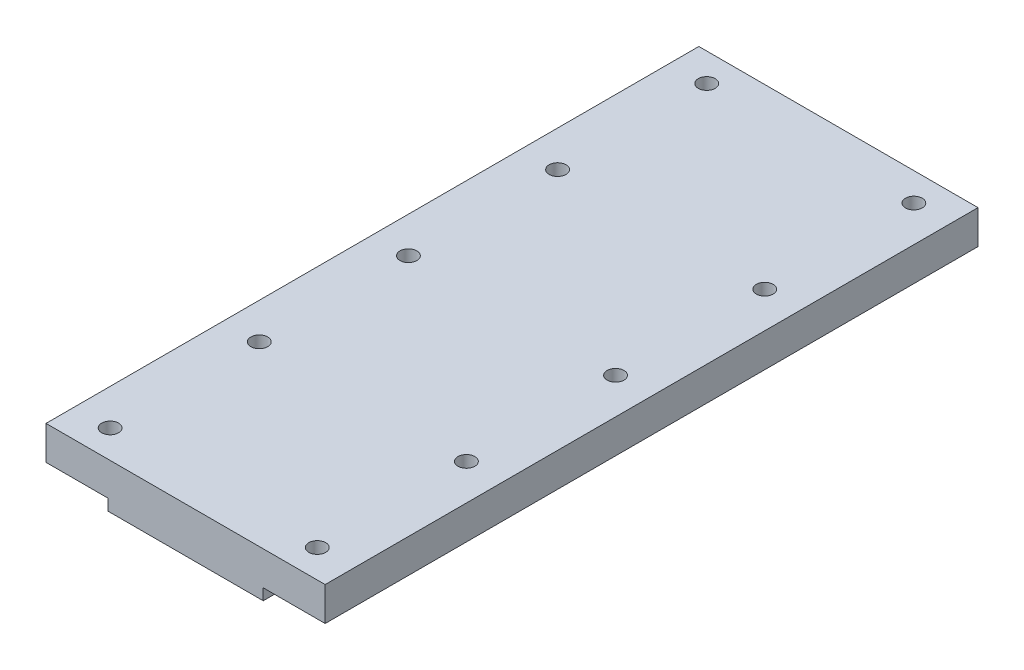
ISO-10303-21;
HEADER;
FILE_DESCRIPTION(('STEP AP214'),'2;1');
FILE_NAME('part.step','',(''),(''),'','','');
FILE_SCHEMA(('AUTOMOTIVE_DESIGN { 1 0 10303 214 1 1 1 1 }'));
ENDSEC;
DATA;
#1=APPLICATION_CONTEXT('core data for automotive mechanical design processes');
#2=APPLICATION_PROTOCOL_DEFINITION('international standard','automotive_design',2000,#1);
#3=PRODUCT_CONTEXT('',#1,'mechanical');
#4=PRODUCT('Part','Part','',(#3));
#5=PRODUCT_RELATED_PRODUCT_CATEGORY('part','',(#4));
#6=PRODUCT_DEFINITION_FORMATION('','',#4);
#7=PRODUCT_DEFINITION_CONTEXT('part definition',#1,'design');
#8=PRODUCT_DEFINITION('design','',#6,#7);
#9=PRODUCT_DEFINITION_SHAPE('','',#8);
#10=(LENGTH_UNIT() NAMED_UNIT(*) SI_UNIT(.MILLI.,.METRE.));
#11=(NAMED_UNIT(*) PLANE_ANGLE_UNIT() SI_UNIT($,.RADIAN.));
#12=(NAMED_UNIT(*) SI_UNIT($,.STERADIAN.) SOLID_ANGLE_UNIT());
#13=UNCERTAINTY_MEASURE_WITH_UNIT(LENGTH_MEASURE(1.E-05),#10,'distance_accuracy_value','');
#14=(GEOMETRIC_REPRESENTATION_CONTEXT(3) GLOBAL_UNCERTAINTY_ASSIGNED_CONTEXT((#13)) GLOBAL_UNIT_ASSIGNED_CONTEXT((#10,
#11,#12)) REPRESENTATION_CONTEXT('',''));
#15=CARTESIAN_POINT('',(0.,0.,0.));
#16=DIRECTION('',(0.,0.,1.));
#17=DIRECTION('',(1.,0.,0.));
#18=AXIS2_PLACEMENT_3D('',#15,#16,#17);
#19=CARTESIAN_POINT('',(-124.,30.,290.));
#20=DIRECTION('',(1.,0.,0.));
#21=DIRECTION('',(0.,0.,-1.));
#22=AXIS2_PLACEMENT_3D('',#19,#20,#21);
#23=PLANE('',#22);
#24=DIRECTION('',(0.,-1.,0.));
#25=VECTOR('',#24,1.);
#26=CARTESIAN_POINT('',(-124.,30.,-290.));
#27=LINE('',#26,#25);
#28=CARTESIAN_POINT('',(-124.,30.,-290.));
#29=VERTEX_POINT('',#28);
#30=CARTESIAN_POINT('',(-124.,0.,-290.));
#31=VERTEX_POINT('',#30);
#32=EDGE_CURVE('E136',#29,#31,#27,.T.);
#33=ORIENTED_EDGE('',*,*,#32,.T.);
#34=DIRECTION('',(0.,0.,-1.));
#35=VECTOR('',#34,1.);
#36=CARTESIAN_POINT('',(-124.,0.,290.));
#37=LINE('',#36,#35);
#38=CARTESIAN_POINT('',(-124.,0.,290.));
#39=VERTEX_POINT('',#38);
#40=EDGE_CURVE('E11',#39,#31,#37,.T.);
#41=ORIENTED_EDGE('',*,*,#40,.F.);
#42=DIRECTION('',(0.,-1.,0.));
#43=VECTOR('',#42,1.);
#44=CARTESIAN_POINT('',(-124.,30.,290.));
#45=LINE('',#44,#43);
#46=CARTESIAN_POINT('',(-124.,30.,290.));
#47=VERTEX_POINT('',#46);
#48=EDGE_CURVE('E155',#47,#39,#45,.T.);
#49=ORIENTED_EDGE('',*,*,#48,.F.);
#50=DIRECTION('',(0.,0.,-1.));
#51=VECTOR('',#50,1.);
#52=CARTESIAN_POINT('',(-124.,30.,290.));
#53=LINE('',#52,#51);
#54=EDGE_CURVE('E134',#47,#29,#53,.T.);
#55=ORIENTED_EDGE('',*,*,#54,.T.);
#56=EDGE_LOOP('',(#33,#41,#49,#55));
#57=FACE_BOUND('',#56,.T.);
#58=ADVANCED_FACE('F39',(#57),#23,.F.);
#59=CARTESIAN_POINT('',(-124.,0.,290.));
#60=DIRECTION('',(0.,1.,0.));
#61=DIRECTION('',(-1.,0.,0.));
#62=AXIS2_PLACEMENT_3D('',#59,#60,#61);
#63=PLANE('',#62);
#64=CARTESIAN_POINT('',(-92.,0.,265.));
#65=DIRECTION('',(0.,1.,0.));
#66=DIRECTION('',(-1.,0.,0.));
#67=AXIS2_PLACEMENT_3D('',#64,#65,#66);
#68=CIRCLE('',#67,7.50000000000001);
#69=CARTESIAN_POINT('',(-99.5,0.,265.));
#70=VERTEX_POINT('',#69);
#71=EDGE_CURVE('E182',#70,#70,#68,.T.);
#72=ORIENTED_EDGE('',*,*,#71,.T.);
#73=EDGE_LOOP('',(#72));
#74=FACE_BOUND('',#73,.T.);
#75=CARTESIAN_POINT('',(-92.,0.,132.5));
#76=DIRECTION('',(0.,1.,0.));
#77=DIRECTION('',(-1.,0.,0.));
#78=AXIS2_PLACEMENT_3D('',#75,#76,#77);
#79=CIRCLE('',#78,7.50000000000001);
#80=CARTESIAN_POINT('',(-99.5,0.,132.5));
#81=VERTEX_POINT('',#80);
#82=EDGE_CURVE('E177',#81,#81,#79,.T.);
#83=ORIENTED_EDGE('',*,*,#82,.T.);
#84=EDGE_LOOP('',(#83));
#85=FACE_BOUND('',#84,.T.);
#86=CARTESIAN_POINT('',(-92.,0.,0.));
#87=DIRECTION('',(0.,1.,0.));
#88=DIRECTION('',(-1.,0.,0.));
#89=AXIS2_PLACEMENT_3D('',#86,#87,#88);
#90=CIRCLE('',#89,7.50000000000001);
#91=CARTESIAN_POINT('',(-99.5,0.,0.));
#92=VERTEX_POINT('',#91);
#93=EDGE_CURVE('E174',#92,#92,#90,.T.);
#94=ORIENTED_EDGE('',*,*,#93,.T.);
#95=EDGE_LOOP('',(#94));
#96=FACE_BOUND('',#95,.T.);
#97=CARTESIAN_POINT('',(-92.,0.,-132.5));
#98=DIRECTION('',(0.,1.,0.));
#99=DIRECTION('',(-1.,0.,0.));
#100=AXIS2_PLACEMENT_3D('',#97,#98,#99);
#101=CIRCLE('',#100,7.50000000000001);
#102=CARTESIAN_POINT('',(-99.5,0.,-132.5));
#103=VERTEX_POINT('',#102);
#104=EDGE_CURVE('E171',#103,#103,#101,.T.);
#105=ORIENTED_EDGE('',*,*,#104,.T.);
#106=EDGE_LOOP('',(#105));
#107=FACE_BOUND('',#106,.T.);
#108=CARTESIAN_POINT('',(-92.,0.,-265.));
#109=DIRECTION('',(0.,1.,0.));
#110=DIRECTION('',(-1.,0.,0.));
#111=AXIS2_PLACEMENT_3D('',#108,#109,#110);
#112=CIRCLE('',#111,7.50000000000001);
#113=CARTESIAN_POINT('',(-99.5,0.,-265.));
#114=VERTEX_POINT('',#113);
#115=EDGE_CURVE('E170',#114,#114,#112,.T.);
#116=ORIENTED_EDGE('',*,*,#115,.T.);
#117=EDGE_LOOP('',(#116));
#118=FACE_BOUND('',#117,.T.);
#119=DIRECTION('',(1.,0.,0.));
#120=VECTOR('',#119,1.);
#121=CARTESIAN_POINT('',(-124.,0.,-290.));
#122=LINE('',#121,#120);
#123=CARTESIAN_POINT('',(-69.,0.,-290.));
#124=VERTEX_POINT('',#123);
#125=EDGE_CURVE('E137',#31,#124,#122,.T.);
#126=ORIENTED_EDGE('',*,*,#125,.T.);
#127=DIRECTION('',(0.,0.,-1.));
#128=VECTOR('',#127,1.);
#129=CARTESIAN_POINT('',(-69.,0.,290.));
#130=LINE('',#129,#128);
#131=CARTESIAN_POINT('',(-69.,0.,290.));
#132=VERTEX_POINT('',#131);
#133=EDGE_CURVE('E48',#132,#124,#130,.T.);
#134=ORIENTED_EDGE('',*,*,#133,.F.);
#135=DIRECTION('',(1.,0.,0.));
#136=VECTOR('',#135,1.);
#137=CARTESIAN_POINT('',(-124.,0.,290.));
#138=LINE('',#137,#136);
#139=EDGE_CURVE('E99',#39,#132,#138,.T.);
#140=ORIENTED_EDGE('',*,*,#139,.F.);
#141=ORIENTED_EDGE('',*,*,#40,.T.);
#142=EDGE_LOOP('',(#126,#134,#140,#141));
#143=FACE_BOUND('',#142,.T.);
#144=ADVANCED_FACE('F247',(#74,#85,#96,#107,#118,#143),#63,.F.);
#145=CARTESIAN_POINT('',(-69.,0.,290.));
#146=DIRECTION('',(1.,0.,0.));
#147=DIRECTION('',(0.,0.,-1.));
#148=AXIS2_PLACEMENT_3D('',#145,#146,#147);
#149=PLANE('',#148);
#150=DIRECTION('',(0.,-1.,0.));
#151=VECTOR('',#150,1.);
#152=CARTESIAN_POINT('',(-69.,0.,-290.));
#153=LINE('',#152,#151);
#154=CARTESIAN_POINT('',(-69.,-9.99999999999998,-290.));
#155=VERTEX_POINT('',#154);
#156=EDGE_CURVE('E141',#124,#155,#153,.T.);
#157=ORIENTED_EDGE('',*,*,#156,.T.);
#158=DIRECTION('',(0.,0.,-1.));
#159=VECTOR('',#158,1.);
#160=CARTESIAN_POINT('',(-69.,-9.99999999999998,290.));
#161=LINE('',#160,#159);
#162=CARTESIAN_POINT('',(-69.,-9.99999999999998,290.));
#163=VERTEX_POINT('',#162);
#164=EDGE_CURVE('E158',#163,#155,#161,.T.);
#165=ORIENTED_EDGE('',*,*,#164,.F.);
#166=DIRECTION('',(0.,-1.,0.));
#167=VECTOR('',#166,1.);
#168=CARTESIAN_POINT('',(-69.,0.,290.));
#169=LINE('',#168,#167);
#170=EDGE_CURVE('E214',#132,#163,#169,.T.);
#171=ORIENTED_EDGE('',*,*,#170,.F.);
#172=ORIENTED_EDGE('',*,*,#133,.T.);
#173=EDGE_LOOP('',(#157,#165,#171,#172));
#174=FACE_BOUND('',#173,.T.);
#175=ADVANCED_FACE('F254',(#174),#149,.F.);
#176=CARTESIAN_POINT('',(-69.,-9.99999999999998,290.));
#177=DIRECTION('',(0.,1.,0.));
#178=DIRECTION('',(-1.,0.,0.));
#179=AXIS2_PLACEMENT_3D('',#176,#177,#178);
#180=PLANE('',#179);
#181=DIRECTION('',(1.,0.,0.));
#182=VECTOR('',#181,1.);
#183=CARTESIAN_POINT('',(-69.,-9.99999999999998,-290.));
#184=LINE('',#183,#182);
#185=CARTESIAN_POINT('',(69.,-10.,-290.));
#186=VERTEX_POINT('',#185);
#187=EDGE_CURVE('E143',#155,#186,#184,.T.);
#188=ORIENTED_EDGE('',*,*,#187,.T.);
#189=DIRECTION('',(0.,0.,-1.));
#190=VECTOR('',#189,1.);
#191=CARTESIAN_POINT('',(69.,-10.,290.));
#192=LINE('',#191,#190);
#193=CARTESIAN_POINT('',(69.,-10.,290.));
#194=VERTEX_POINT('',#193);
#195=EDGE_CURVE('E159',#194,#186,#192,.T.);
#196=ORIENTED_EDGE('',*,*,#195,.F.);
#197=DIRECTION('',(1.,0.,0.));
#198=VECTOR('',#197,1.);
#199=CARTESIAN_POINT('',(-69.,-9.99999999999998,290.));
#200=LINE('',#199,#198);
#201=EDGE_CURVE('E213',#163,#194,#200,.T.);
#202=ORIENTED_EDGE('',*,*,#201,.F.);
#203=ORIENTED_EDGE('',*,*,#164,.T.);
#204=EDGE_LOOP('',(#188,#196,#202,#203));
#205=FACE_BOUND('',#204,.T.);
#206=ADVANCED_FACE('F224',(#205),#180,.F.);
#207=CARTESIAN_POINT('',(69.,-10.,290.));
#208=DIRECTION('',(-1.,0.,0.));
#209=DIRECTION('',(0.,0.,1.));
#210=AXIS2_PLACEMENT_3D('',#207,#208,#209);
#211=PLANE('',#210);
#212=DIRECTION('',(0.,1.,0.));
#213=VECTOR('',#212,1.);
#214=CARTESIAN_POINT('',(69.,-10.,-290.));
#215=LINE('',#214,#213);
#216=CARTESIAN_POINT('',(69.,0.,-290.));
#217=VERTEX_POINT('',#216);
#218=EDGE_CURVE('E150',#186,#217,#215,.T.);
#219=ORIENTED_EDGE('',*,*,#218,.T.);
#220=DIRECTION('',(0.,0.,-1.));
#221=VECTOR('',#220,1.);
#222=CARTESIAN_POINT('',(69.,0.,290.));
#223=LINE('',#222,#221);
#224=CARTESIAN_POINT('',(69.,0.,290.));
#225=VERTEX_POINT('',#224);
#226=EDGE_CURVE('E129',#225,#217,#223,.T.);
#227=ORIENTED_EDGE('',*,*,#226,.F.);
#228=DIRECTION('',(0.,1.,0.));
#229=VECTOR('',#228,1.);
#230=CARTESIAN_POINT('',(69.,-10.,290.));
#231=LINE('',#230,#229);
#232=EDGE_CURVE('E118',#194,#225,#231,.T.);
#233=ORIENTED_EDGE('',*,*,#232,.F.);
#234=ORIENTED_EDGE('',*,*,#195,.T.);
#235=EDGE_LOOP('',(#219,#227,#233,#234));
#236=FACE_BOUND('',#235,.T.);
#237=ADVANCED_FACE('F222',(#236),#211,.F.);
#238=CARTESIAN_POINT('',(69.,0.,290.));
#239=DIRECTION('',(0.,1.,0.));
#240=DIRECTION('',(0.,0.,1.));
#241=AXIS2_PLACEMENT_3D('',#238,#239,#240);
#242=PLANE('',#241);
#243=CARTESIAN_POINT('',(92.,0.,-265.));
#244=DIRECTION('',(0.,1.,0.));
#245=DIRECTION('',(0.,0.,1.));
#246=AXIS2_PLACEMENT_3D('',#243,#244,#245);
#247=CIRCLE('',#246,7.50000000000001);
#248=CARTESIAN_POINT('',(92.,0.,-257.5));
#249=VERTEX_POINT('',#248);
#250=EDGE_CURVE('E142',#249,#249,#247,.T.);
#251=ORIENTED_EDGE('',*,*,#250,.T.);
#252=EDGE_LOOP('',(#251));
#253=FACE_BOUND('',#252,.T.);
#254=CARTESIAN_POINT('',(92.,0.,265.));
#255=DIRECTION('',(0.,1.,0.));
#256=DIRECTION('',(0.,0.,1.));
#257=AXIS2_PLACEMENT_3D('',#254,#255,#256);
#258=CIRCLE('',#257,7.50000000000001);
#259=CARTESIAN_POINT('',(92.,0.,272.5));
#260=VERTEX_POINT('',#259);
#261=EDGE_CURVE('E200',#260,#260,#258,.T.);
#262=ORIENTED_EDGE('',*,*,#261,.T.);
#263=EDGE_LOOP('',(#262));
#264=FACE_BOUND('',#263,.T.);
#265=CARTESIAN_POINT('',(92.,0.,132.5));
#266=DIRECTION('',(0.,1.,0.));
#267=DIRECTION('',(0.,0.,1.));
#268=AXIS2_PLACEMENT_3D('',#265,#266,#267);
#269=CIRCLE('',#268,7.50000000000001);
#270=CARTESIAN_POINT('',(92.,0.,140.));
#271=VERTEX_POINT('',#270);
#272=EDGE_CURVE('E191',#271,#271,#269,.T.);
#273=ORIENTED_EDGE('',*,*,#272,.T.);
#274=EDGE_LOOP('',(#273));
#275=FACE_BOUND('',#274,.T.);
#276=CARTESIAN_POINT('',(92.,0.,0.));
#277=DIRECTION('',(0.,1.,0.));
#278=DIRECTION('',(0.,0.,1.));
#279=AXIS2_PLACEMENT_3D('',#276,#277,#278);
#280=CIRCLE('',#279,7.50000000000001);
#281=CARTESIAN_POINT('',(92.,0.,7.50000000000007));
#282=VERTEX_POINT('',#281);
#283=EDGE_CURVE('E192',#282,#282,#280,.T.);
#284=ORIENTED_EDGE('',*,*,#283,.T.);
#285=EDGE_LOOP('',(#284));
#286=FACE_BOUND('',#285,.T.);
#287=CARTESIAN_POINT('',(92.,0.,-132.5));
#288=DIRECTION('',(0.,1.,0.));
#289=DIRECTION('',(0.,0.,1.));
#290=AXIS2_PLACEMENT_3D('',#287,#288,#289);
#291=CIRCLE('',#290,7.50000000000001);
#292=CARTESIAN_POINT('',(92.,0.,-125.));
#293=VERTEX_POINT('',#292);
#294=EDGE_CURVE('E190',#293,#293,#291,.T.);
#295=ORIENTED_EDGE('',*,*,#294,.T.);
#296=EDGE_LOOP('',(#295));
#297=FACE_BOUND('',#296,.T.);
#298=DIRECTION('',(1.,0.,0.));
#299=VECTOR('',#298,1.);
#300=CARTESIAN_POINT('',(69.,0.,-290.));
#301=LINE('',#300,#299);
#302=CARTESIAN_POINT('',(124.,0.,-290.));
#303=VERTEX_POINT('',#302);
#304=EDGE_CURVE('E130',#217,#303,#301,.T.);
#305=ORIENTED_EDGE('',*,*,#304,.T.);
#306=DIRECTION('',(0.,0.,-1.));
#307=VECTOR('',#306,1.);
#308=CARTESIAN_POINT('',(124.,0.,290.));
#309=LINE('',#308,#307);
#310=CARTESIAN_POINT('',(124.,0.,290.));
#311=VERTEX_POINT('',#310);
#312=EDGE_CURVE('E121',#311,#303,#309,.T.);
#313=ORIENTED_EDGE('',*,*,#312,.F.);
#314=DIRECTION('',(1.,0.,0.));
#315=VECTOR('',#314,1.);
#316=CARTESIAN_POINT('',(69.,0.,290.));
#317=LINE('',#316,#315);
#318=EDGE_CURVE('E113',#225,#311,#317,.T.);
#319=ORIENTED_EDGE('',*,*,#318,.F.);
#320=ORIENTED_EDGE('',*,*,#226,.T.);
#321=EDGE_LOOP('',(#305,#313,#319,#320));
#322=FACE_BOUND('',#321,.T.);
#323=ADVANCED_FACE('F123',(#253,#264,#275,#286,#297,#322),#242,.F.);
#324=CARTESIAN_POINT('',(124.,0.,290.));
#325=DIRECTION('',(-1.,0.,0.));
#326=DIRECTION('',(0.,0.,1.));
#327=AXIS2_PLACEMENT_3D('',#324,#325,#326);
#328=PLANE('',#327);
#329=DIRECTION('',(0.,1.,0.));
#330=VECTOR('',#329,1.);
#331=CARTESIAN_POINT('',(124.,0.,-290.));
#332=LINE('',#331,#330);
#333=CARTESIAN_POINT('',(124.,30.,-290.));
#334=VERTEX_POINT('',#333);
#335=EDGE_CURVE('E87',#303,#334,#332,.T.);
#336=ORIENTED_EDGE('',*,*,#335,.T.);
#337=DIRECTION('',(0.,0.,-1.));
#338=VECTOR('',#337,1.);
#339=CARTESIAN_POINT('',(124.,30.,290.));
#340=LINE('',#339,#338);
#341=CARTESIAN_POINT('',(124.,30.,290.));
#342=VERTEX_POINT('',#341);
#343=EDGE_CURVE('E126',#342,#334,#340,.T.);
#344=ORIENTED_EDGE('',*,*,#343,.F.);
#345=DIRECTION('',(0.,1.,0.));
#346=VECTOR('',#345,1.);
#347=CARTESIAN_POINT('',(124.,0.,290.));
#348=LINE('',#347,#346);
#349=EDGE_CURVE('E120',#311,#342,#348,.T.);
#350=ORIENTED_EDGE('',*,*,#349,.F.);
#351=ORIENTED_EDGE('',*,*,#312,.T.);
#352=EDGE_LOOP('',(#336,#344,#350,#351));
#353=FACE_BOUND('',#352,.T.);
#354=ADVANCED_FACE('F132',(#353),#328,.F.);
#355=CARTESIAN_POINT('',(124.,30.,290.));
#356=DIRECTION('',(0.,-1.,0.));
#357=DIRECTION('',(1.,0.,0.));
#358=AXIS2_PLACEMENT_3D('',#355,#356,#357);
#359=PLANE('',#358);
#360=CARTESIAN_POINT('',(92.,30.,-265.));
#361=DIRECTION('',(0.,-1.,0.));
#362=DIRECTION('',(1.,0.,0.));
#363=AXIS2_PLACEMENT_3D('',#360,#361,#362);
#364=CIRCLE('',#363,7.50000000000001);
#365=CARTESIAN_POINT('',(99.5,30.,-265.));
#366=VERTEX_POINT('',#365);
#367=EDGE_CURVE('E45',#366,#366,#364,.T.);
#368=ORIENTED_EDGE('',*,*,#367,.T.);
#369=EDGE_LOOP('',(#368));
#370=FACE_BOUND('',#369,.T.);
#371=CARTESIAN_POINT('',(92.,30.,265.));
#372=DIRECTION('',(0.,-1.,0.));
#373=DIRECTION('',(1.,0.,0.));
#374=AXIS2_PLACEMENT_3D('',#371,#372,#373);
#375=CIRCLE('',#374,7.50000000000001);
#376=CARTESIAN_POINT('',(99.5,30.,265.));
#377=VERTEX_POINT('',#376);
#378=EDGE_CURVE('E193',#377,#377,#375,.T.);
#379=ORIENTED_EDGE('',*,*,#378,.T.);
#380=EDGE_LOOP('',(#379));
#381=FACE_BOUND('',#380,.T.);
#382=CARTESIAN_POINT('',(92.,30.,132.5));
#383=DIRECTION('',(0.,-1.,0.));
#384=DIRECTION('',(1.,0.,0.));
#385=AXIS2_PLACEMENT_3D('',#382,#383,#384);
#386=CIRCLE('',#385,7.50000000000001);
#387=CARTESIAN_POINT('',(99.5,30.,132.5));
#388=VERTEX_POINT('',#387);
#389=EDGE_CURVE('E195',#388,#388,#386,.T.);
#390=ORIENTED_EDGE('',*,*,#389,.T.);
#391=EDGE_LOOP('',(#390));
#392=FACE_BOUND('',#391,.T.);
#393=CARTESIAN_POINT('',(92.,30.,0.));
#394=DIRECTION('',(0.,-1.,0.));
#395=DIRECTION('',(1.,0.,0.));
#396=AXIS2_PLACEMENT_3D('',#393,#394,#395);
#397=CIRCLE('',#396,7.50000000000001);
#398=CARTESIAN_POINT('',(99.5,30.,0.));
#399=VERTEX_POINT('',#398);
#400=EDGE_CURVE('E189',#399,#399,#397,.T.);
#401=ORIENTED_EDGE('',*,*,#400,.T.);
#402=EDGE_LOOP('',(#401));
#403=FACE_BOUND('',#402,.T.);
#404=CARTESIAN_POINT('',(92.,30.,-132.5));
#405=DIRECTION('',(0.,-1.,0.));
#406=DIRECTION('',(1.,0.,0.));
#407=AXIS2_PLACEMENT_3D('',#404,#405,#406);
#408=CIRCLE('',#407,7.50000000000001);
#409=CARTESIAN_POINT('',(99.5,30.,-132.5));
#410=VERTEX_POINT('',#409);
#411=EDGE_CURVE('E183',#410,#410,#408,.T.);
#412=ORIENTED_EDGE('',*,*,#411,.T.);
#413=EDGE_LOOP('',(#412));
#414=FACE_BOUND('',#413,.T.);
#415=CARTESIAN_POINT('',(-92.,29.9999999999999,265.));
#416=DIRECTION('',(0.,-1.,0.));
#417=DIRECTION('',(1.,0.,0.));
#418=AXIS2_PLACEMENT_3D('',#415,#416,#417);
#419=CIRCLE('',#418,7.50000000000001);
#420=CARTESIAN_POINT('',(-84.5,29.9999999999999,265.));
#421=VERTEX_POINT('',#420);
#422=EDGE_CURVE('E179',#421,#421,#419,.T.);
#423=ORIENTED_EDGE('',*,*,#422,.T.);
#424=EDGE_LOOP('',(#423));
#425=FACE_BOUND('',#424,.T.);
#426=CARTESIAN_POINT('',(-92.,29.9999999999999,132.5));
#427=DIRECTION('',(0.,-1.,0.));
#428=DIRECTION('',(1.,0.,0.));
#429=AXIS2_PLACEMENT_3D('',#426,#427,#428);
#430=CIRCLE('',#429,7.50000000000001);
#431=CARTESIAN_POINT('',(-84.5,29.9999999999999,132.5));
#432=VERTEX_POINT('',#431);
#433=EDGE_CURVE('E176',#432,#432,#430,.T.);
#434=ORIENTED_EDGE('',*,*,#433,.T.);
#435=EDGE_LOOP('',(#434));
#436=FACE_BOUND('',#435,.T.);
#437=CARTESIAN_POINT('',(-92.,29.9999999999999,0.));
#438=DIRECTION('',(0.,-1.,0.));
#439=DIRECTION('',(1.,0.,0.));
#440=AXIS2_PLACEMENT_3D('',#437,#438,#439);
#441=CIRCLE('',#440,7.50000000000001);
#442=CARTESIAN_POINT('',(-84.5,29.9999999999999,0.));
#443=VERTEX_POINT('',#442);
#444=EDGE_CURVE('E175',#443,#443,#441,.T.);
#445=ORIENTED_EDGE('',*,*,#444,.T.);
#446=EDGE_LOOP('',(#445));
#447=FACE_BOUND('',#446,.T.);
#448=CARTESIAN_POINT('',(-92.,29.9999999999999,-132.5));
#449=DIRECTION('',(0.,-1.,0.));
#450=DIRECTION('',(1.,0.,0.));
#451=AXIS2_PLACEMENT_3D('',#448,#449,#450);
#452=CIRCLE('',#451,7.50000000000001);
#453=CARTESIAN_POINT('',(-84.5,29.9999999999999,-132.5));
#454=VERTEX_POINT('',#453);
#455=EDGE_CURVE('E166',#454,#454,#452,.T.);
#456=ORIENTED_EDGE('',*,*,#455,.T.);
#457=EDGE_LOOP('',(#456));
#458=FACE_BOUND('',#457,.T.);
#459=CARTESIAN_POINT('',(-92.,29.9999999999999,-265.));
#460=DIRECTION('',(0.,-1.,0.));
#461=DIRECTION('',(1.,0.,0.));
#462=AXIS2_PLACEMENT_3D('',#459,#460,#461);
#463=CIRCLE('',#462,7.50000000000001);
#464=CARTESIAN_POINT('',(-84.5,29.9999999999999,-265.));
#465=VERTEX_POINT('',#464);
#466=EDGE_CURVE('E165',#465,#465,#463,.T.);
#467=ORIENTED_EDGE('',*,*,#466,.T.);
#468=EDGE_LOOP('',(#467));
#469=FACE_BOUND('',#468,.T.);
#470=DIRECTION('',(-1.,0.,0.));
#471=VECTOR('',#470,1.);
#472=CARTESIAN_POINT('',(124.,30.,-290.));
#473=LINE('',#472,#471);
#474=EDGE_CURVE('E91',#334,#29,#473,.T.);
#475=ORIENTED_EDGE('',*,*,#474,.T.);
#476=ORIENTED_EDGE('',*,*,#54,.F.);
#477=DIRECTION('',(-1.,0.,0.));
#478=VECTOR('',#477,1.);
#479=CARTESIAN_POINT('',(124.,30.,290.));
#480=LINE('',#479,#478);
#481=EDGE_CURVE('E60',#342,#47,#480,.T.);
#482=ORIENTED_EDGE('',*,*,#481,.F.);
#483=ORIENTED_EDGE('',*,*,#343,.T.);
#484=EDGE_LOOP('',(#475,#476,#482,#483));
#485=FACE_BOUND('',#484,.T.);
#486=ADVANCED_FACE('F231',(#370,#381,#392,#403,#414,#425,#436,#447,#458,#469,#485),#359,.F.);
#487=CARTESIAN_POINT('',(0.,0.,290.));
#488=DIRECTION('',(0.,0.,1.));
#489=DIRECTION('',(1.,0.,0.));
#490=AXIS2_PLACEMENT_3D('',#487,#488,#489);
#491=PLANE('',#490);
#492=ORIENTED_EDGE('',*,*,#48,.T.);
#493=ORIENTED_EDGE('',*,*,#139,.T.);
#494=ORIENTED_EDGE('',*,*,#170,.T.);
#495=ORIENTED_EDGE('',*,*,#201,.T.);
#496=ORIENTED_EDGE('',*,*,#232,.T.);
#497=ORIENTED_EDGE('',*,*,#318,.T.);
#498=ORIENTED_EDGE('',*,*,#349,.T.);
#499=ORIENTED_EDGE('',*,*,#481,.T.);
#500=EDGE_LOOP('',(#492,#493,#494,#495,#496,#497,#498,#499));
#501=FACE_BOUND('',#500,.T.);
#502=ADVANCED_FACE('F114',(#501),#491,.T.);
#503=CARTESIAN_POINT('',(0.,0.,-290.));
#504=DIRECTION('',(0.,0.,1.));
#505=DIRECTION('',(1.,0.,0.));
#506=AXIS2_PLACEMENT_3D('',#503,#504,#505);
#507=PLANE('',#506);
#508=ORIENTED_EDGE('',*,*,#32,.F.);
#509=ORIENTED_EDGE('',*,*,#474,.F.);
#510=ORIENTED_EDGE('',*,*,#335,.F.);
#511=ORIENTED_EDGE('',*,*,#304,.F.);
#512=ORIENTED_EDGE('',*,*,#218,.F.);
#513=ORIENTED_EDGE('',*,*,#187,.F.);
#514=ORIENTED_EDGE('',*,*,#156,.F.);
#515=ORIENTED_EDGE('',*,*,#125,.F.);
#516=EDGE_LOOP('',(#508,#509,#510,#511,#512,#513,#514,#515));
#517=FACE_BOUND('',#516,.T.);
#518=ADVANCED_FACE('F226',(#517),#507,.F.);
#519=CARTESIAN_POINT('',(-92.,-260.,-265.));
#520=DIRECTION('',(0.,1.,0.));
#521=DIRECTION('',(-1.,0.,0.));
#522=AXIS2_PLACEMENT_3D('',#519,#520,#521);
#523=CYLINDRICAL_SURFACE('',#522,7.50000000000001);
#524=ORIENTED_EDGE('',*,*,#466,.F.);
#525=EDGE_LOOP('',(#524));
#526=FACE_BOUND('',#525,.T.);
#527=ORIENTED_EDGE('',*,*,#115,.F.);
#528=EDGE_LOOP('',(#527));
#529=FACE_BOUND('',#528,.T.);
#530=ADVANCED_FACE('F292',(#526,#529),#523,.F.);
#531=CARTESIAN_POINT('',(-92.,-260.,-132.5));
#532=DIRECTION('',(0.,1.,0.));
#533=DIRECTION('',(-1.,0.,0.));
#534=AXIS2_PLACEMENT_3D('',#531,#532,#533);
#535=CYLINDRICAL_SURFACE('',#534,7.50000000000001);
#536=ORIENTED_EDGE('',*,*,#455,.F.);
#537=EDGE_LOOP('',(#536));
#538=FACE_BOUND('',#537,.T.);
#539=ORIENTED_EDGE('',*,*,#104,.F.);
#540=EDGE_LOOP('',(#539));
#541=FACE_BOUND('',#540,.T.);
#542=ADVANCED_FACE('F291',(#538,#541),#535,.F.);
#543=CARTESIAN_POINT('',(-92.,-260.,0.));
#544=DIRECTION('',(0.,1.,0.));
#545=DIRECTION('',(-1.,0.,0.));
#546=AXIS2_PLACEMENT_3D('',#543,#544,#545);
#547=CYLINDRICAL_SURFACE('',#546,7.50000000000001);
#548=ORIENTED_EDGE('',*,*,#444,.F.);
#549=EDGE_LOOP('',(#548));
#550=FACE_BOUND('',#549,.T.);
#551=ORIENTED_EDGE('',*,*,#93,.F.);
#552=EDGE_LOOP('',(#551));
#553=FACE_BOUND('',#552,.T.);
#554=ADVANCED_FACE('F299',(#550,#553),#547,.F.);
#555=CARTESIAN_POINT('',(-92.,-260.,132.5));
#556=DIRECTION('',(0.,1.,0.));
#557=DIRECTION('',(-1.,0.,0.));
#558=AXIS2_PLACEMENT_3D('',#555,#556,#557);
#559=CYLINDRICAL_SURFACE('',#558,7.50000000000001);
#560=ORIENTED_EDGE('',*,*,#433,.F.);
#561=EDGE_LOOP('',(#560));
#562=FACE_BOUND('',#561,.T.);
#563=ORIENTED_EDGE('',*,*,#82,.F.);
#564=EDGE_LOOP('',(#563));
#565=FACE_BOUND('',#564,.T.);
#566=ADVANCED_FACE('F330',(#562,#565),#559,.F.);
#567=CARTESIAN_POINT('',(-92.,-260.,265.));
#568=DIRECTION('',(0.,1.,0.));
#569=DIRECTION('',(-1.,0.,0.));
#570=AXIS2_PLACEMENT_3D('',#567,#568,#569);
#571=CYLINDRICAL_SURFACE('',#570,7.50000000000001);
#572=ORIENTED_EDGE('',*,*,#422,.F.);
#573=EDGE_LOOP('',(#572));
#574=FACE_BOUND('',#573,.T.);
#575=ORIENTED_EDGE('',*,*,#71,.F.);
#576=EDGE_LOOP('',(#575));
#577=FACE_BOUND('',#576,.T.);
#578=ADVANCED_FACE('F324',(#574,#577),#571,.F.);
#579=CARTESIAN_POINT('',(92.,-260.,-132.5));
#580=DIRECTION('',(0.,1.,0.));
#581=DIRECTION('',(-1.,0.,0.));
#582=AXIS2_PLACEMENT_3D('',#579,#580,#581);
#583=CYLINDRICAL_SURFACE('',#582,7.50000000000001);
#584=ORIENTED_EDGE('',*,*,#411,.F.);
#585=EDGE_LOOP('',(#584));
#586=FACE_BOUND('',#585,.T.);
#587=ORIENTED_EDGE('',*,*,#294,.F.);
#588=EDGE_LOOP('',(#587));
#589=FACE_BOUND('',#588,.T.);
#590=ADVANCED_FACE('F316',(#586,#589),#583,.F.);
#591=CARTESIAN_POINT('',(92.,-260.,0.));
#592=DIRECTION('',(0.,1.,0.));
#593=DIRECTION('',(-1.,0.,0.));
#594=AXIS2_PLACEMENT_3D('',#591,#592,#593);
#595=CYLINDRICAL_SURFACE('',#594,7.50000000000001);
#596=ORIENTED_EDGE('',*,*,#400,.F.);
#597=EDGE_LOOP('',(#596));
#598=FACE_BOUND('',#597,.T.);
#599=ORIENTED_EDGE('',*,*,#283,.F.);
#600=EDGE_LOOP('',(#599));
#601=FACE_BOUND('',#600,.T.);
#602=ADVANCED_FACE('F314',(#598,#601),#595,.F.);
#603=CARTESIAN_POINT('',(92.,-260.,132.5));
#604=DIRECTION('',(0.,1.,0.));
#605=DIRECTION('',(-1.,0.,0.));
#606=AXIS2_PLACEMENT_3D('',#603,#604,#605);
#607=CYLINDRICAL_SURFACE('',#606,7.50000000000001);
#608=ORIENTED_EDGE('',*,*,#389,.F.);
#609=EDGE_LOOP('',(#608));
#610=FACE_BOUND('',#609,.T.);
#611=ORIENTED_EDGE('',*,*,#272,.F.);
#612=EDGE_LOOP('',(#611));
#613=FACE_BOUND('',#612,.T.);
#614=ADVANCED_FACE('F311',(#610,#613),#607,.F.);
#615=CARTESIAN_POINT('',(92.,-260.,265.));
#616=DIRECTION('',(0.,1.,0.));
#617=DIRECTION('',(-1.,0.,0.));
#618=AXIS2_PLACEMENT_3D('',#615,#616,#617);
#619=CYLINDRICAL_SURFACE('',#618,7.50000000000001);
#620=ORIENTED_EDGE('',*,*,#378,.F.);
#621=EDGE_LOOP('',(#620));
#622=FACE_BOUND('',#621,.T.);
#623=ORIENTED_EDGE('',*,*,#261,.F.);
#624=EDGE_LOOP('',(#623));
#625=FACE_BOUND('',#624,.T.);
#626=ADVANCED_FACE('F310',(#622,#625),#619,.F.);
#627=CARTESIAN_POINT('',(92.,-260.,-265.));
#628=DIRECTION('',(0.,1.,0.));
#629=DIRECTION('',(-1.,0.,0.));
#630=AXIS2_PLACEMENT_3D('',#627,#628,#629);
#631=CYLINDRICAL_SURFACE('',#630,7.50000000000001);
#632=ORIENTED_EDGE('',*,*,#367,.F.);
#633=EDGE_LOOP('',(#632));
#634=FACE_BOUND('',#633,.T.);
#635=ORIENTED_EDGE('',*,*,#250,.F.);
#636=EDGE_LOOP('',(#635));
#637=FACE_BOUND('',#636,.T.);
#638=ADVANCED_FACE('F302',(#634,#637),#631,.F.);
#639=CLOSED_SHELL('',(#58,#144,#175,#206,#237,#323,#354,#486,#502,#518,#530,#542,#554,#566,#578,
#590,#602,#614,#626,#638));
#640=MANIFOLD_SOLID_BREP('B2',#639);
#641=ADVANCED_BREP_SHAPE_REPRESENTATION('',(#18,#640),#14);
#642=SHAPE_DEFINITION_REPRESENTATION(#9,#641);
ENDSEC;
END-ISO-10303-21;
